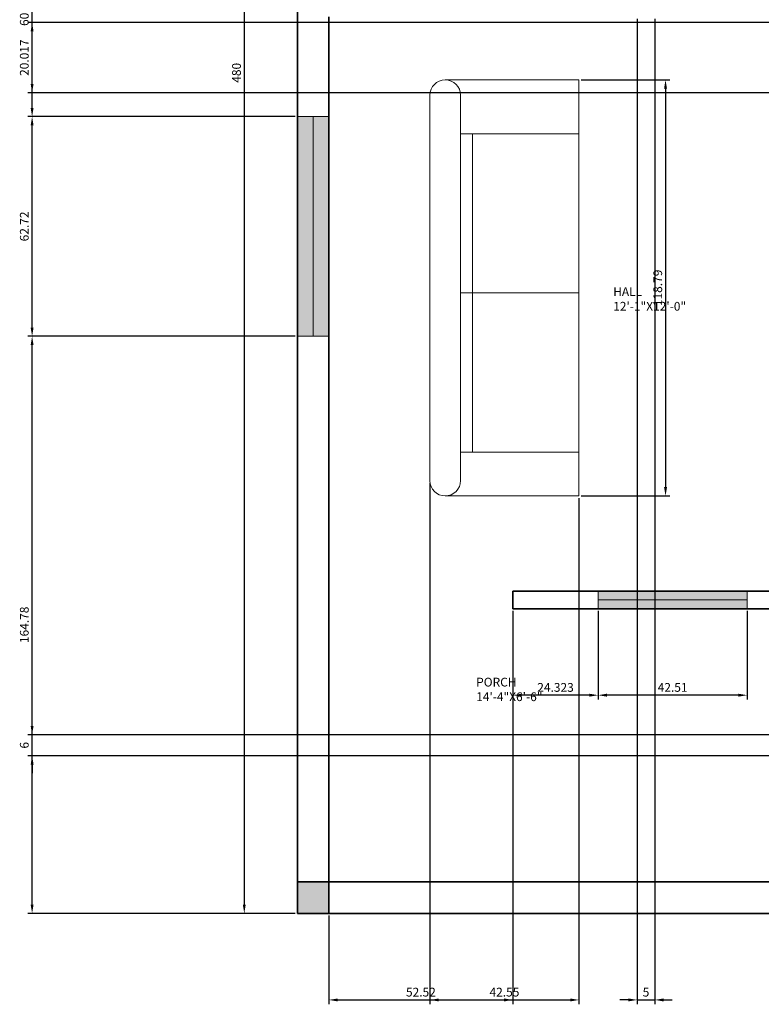
# Model space of a CAD drawing. Units: inches. Extents: x 33934 to 34340, y 20959 to 21493.
# Tile 1 of 4: x 33934 to 34146, y 20959 to 21240. Entities that reach past the tile are written whole.
import ezdxf

# ---------------------------------------------------------------- set-up
doc = ezdxf.new("R2010")
doc.units = ezdxf.units.IN
for name, color, linetype, lineweight in [('A-ANNO-DIMS', 2, 'Continuous', 18), ('A-AREA-IDEN', 7, 'Continuous', 18), ('A-FURN', 8, 'Continuous', 18), ('A-GLAZ', 4, 'Continuous', 18), ('A-WALL', 7, 'Continuous', 35)]:
    doc.layers.add(name, color=color, linetype=linetype, lineweight=lineweight)
doc.layers.add('A-COLS-PATT', color=141, linetype='Continuous', lineweight=13, true_color=0xadddf7)
doc.layers.add('A-GLAZ-PATT', color=159, linetype='Continuous', lineweight=13, true_color=0x22346e)
doc.styles.get("Standard").update_dxf_attribs({"font": 'arial.ttf'})
doc.dimstyles.new('ISO-25', dxfattribs={"dimtxt": 2.5, "dimasz": 2.5, "dimexe": 1.25, "dimexo": 0.625, "dimtad": 1, "dimtxsty": 'Standard', "dimcen": 2.5, "dimadec": 0, "dimazin": 0, "dimtfac": 1, "dimtmove": 0, "dimatfit": 3, "dimfxl": 1, "dimarcsym": 0})

# ---------------------------------------------------------------- blocks, each defined once
blk = doc.blocks.new('*D7')
at = {"layer": 'A-ANNO-DIMS', "color": 0, "lineweight": -2, "transparency": 16777216}
for p, q in [((34013.07, 21465.11), (33997.3, 21465.11)), ((33998.55, 21462.61), (33998.55, 20987.61)), ((34013.07, 20985.11), (33997.3, 20985.11))]:
    blk.add_line(p, q, dxfattribs=at)
at = {"layer": 'A-ANNO-DIMS', "color": 0, "transparency": 16777216}
for points in [[(33998.13, 21462.61), (33998.96, 21462.61), (33998.55, 21465.11)], [(33998.13, 20987.61), (33998.96, 20987.61), (33998.55, 20985.11)]]:
    blk.add_solid(points, dxfattribs=at)
at = {"layer": 'Defpoints', "color": 0, "transparency": 16777216}
for p in [(34013.69, 21465.11), (33998.55, 20985.11), (34013.69, 20985.11)]:
    blk.add_point(p, dxfattribs=at)
at = {"layer": 'A-ANNO-DIMS', "color": 0, "transparency": 16777216, "insert": (33996.64, 21225.11), "char_height": 2.5, "attachment_point": 5, "rotation": 90}
blk.add_mtext('480', dxfattribs=at)
blk = doc.blocks.new('*D17')
at = {"layer": 'A-ANNO-DIMS', "color": 0, "lineweight": -2, "transparency": 16777216}
for p, q in [((34013.07, 21149.89), (33936.74, 21149.89)), ((33937.99, 20987.61), (33937.99, 21147.39)), ((34013.07, 20985.11), (33936.74, 20985.11))]:
    blk.add_line(p, q, dxfattribs=at)
at = {"layer": 'A-ANNO-DIMS', "color": 0, "transparency": 16777216}
for points in [[(33937.58, 21147.39), (33938.41, 21147.39), (33937.99, 21149.89)], [(33937.58, 20987.61), (33938.41, 20987.61), (33937.99, 20985.11)]]:
    blk.add_solid(points, dxfattribs=at)
at = {"layer": 'Defpoints', "color": 0, "transparency": 16777216}
for p in [(33937.99, 21149.89), (34013.69, 21149.89), (34013.69, 20985.11)]:
    blk.add_point(p, dxfattribs=at)
at = {"layer": 'A-ANNO-DIMS', "color": 0, "transparency": 16777216, "insert": (33936.09, 21067.5), "char_height": 2.5, "attachment_point": 5, "rotation": 90}
blk.add_mtext('164.78', dxfattribs=at)
blk = doc.blocks.new('*D18')
at = {"layer": 'A-ANNO-DIMS', "color": 0, "lineweight": -2, "transparency": 16777216}
for p, q in [((34013.07, 21212.61), (33936.74, 21212.61)), ((33937.99, 21152.39), (33937.99, 21210.11)), ((34013.07, 21149.89), (33936.74, 21149.89))]:
    blk.add_line(p, q, dxfattribs=at)
at = {"layer": 'A-ANNO-DIMS', "color": 0, "transparency": 16777216}
for points in [[(33937.58, 21210.11), (33938.41, 21210.11), (33937.99, 21212.61)], [(33937.58, 21152.39), (33938.41, 21152.39), (33937.99, 21149.89)]]:
    blk.add_solid(points, dxfattribs=at)
at = {"layer": 'Defpoints', "color": 0, "transparency": 16777216}
for p in [(33937.99, 21212.61), (34013.69, 21212.61), (34013.69, 21149.89)]:
    blk.add_point(p, dxfattribs=at)
at = {"layer": 'A-ANNO-DIMS', "color": 0, "transparency": 16777216, "insert": (33936.09, 21181.25), "char_height": 2.5, "attachment_point": 5, "rotation": 90}
blk.add_mtext('62.72', dxfattribs=at)
blk = doc.blocks.new('*D19')
at = {"layer": 'A-ANNO-DIMS', "color": 0, "lineweight": -2, "transparency": 16777216}
for p, q in [((34013.07, 21272.89), (33936.74, 21272.89)), ((33937.99, 21215.11), (33937.99, 21270.39)), ((34013.07, 21212.61), (33936.74, 21212.61))]:
    blk.add_line(p, q, dxfattribs=at)
at = {"layer": 'A-ANNO-DIMS', "color": 0, "transparency": 16777216}
for points in [[(33937.58, 21270.39), (33938.41, 21270.39), (33937.99, 21272.89)], [(33937.58, 21215.11), (33938.41, 21215.11), (33937.99, 21212.61)]]:
    blk.add_solid(points, dxfattribs=at)
at = {"layer": 'Defpoints', "color": 0, "transparency": 16777216}
for p in [(33937.99, 21272.89), (34013.69, 21272.89), (34013.69, 21212.61)]:
    blk.add_point(p, dxfattribs=at)
at = {"layer": 'A-ANNO-DIMS', "color": 0, "transparency": 16777216, "insert": (33936.09, 21242.75), "char_height": 2.5, "attachment_point": 5, "rotation": 90}
blk.add_mtext('60.28', dxfattribs=at)
blk = doc.blocks.new('*D32')
at = {"layer": 'A-ANNO-DIMS', "color": 0, "lineweight": -2, "transparency": 16777216}
for p, q in [((33937.99, 21038.61), (33937.99, 21041.11)), ((34167.07, 21036.11), (33936.74, 21036.11)), ((33937.99, 21030.11), (33937.99, 21036.11)), ((34167.07, 21030.11), (33936.74, 21030.11)), ((33937.99, 21027.61), (33937.99, 21025.11))]:
    blk.add_line(p, q, dxfattribs=at)
at = {"layer": 'A-ANNO-DIMS', "color": 0, "transparency": 16777216}
for points in [[(33937.58, 21038.61), (33938.41, 21038.61), (33937.99, 21036.11)], [(33937.58, 21027.61), (33938.41, 21027.61), (33937.99, 21030.11)]]:
    blk.add_solid(points, dxfattribs=at)
at = {"layer": 'Defpoints', "color": 0, "transparency": 16777216}
for p in [(33937.99, 21036.11), (34167.69, 21036.11), (34167.69, 21030.11)]:
    blk.add_point(p, dxfattribs=at)
at = {"layer": 'A-ANNO-DIMS', "color": 0, "transparency": 16777216, "insert": (33936.09, 21033.11), "char_height": 2.5, "attachment_point": 5, "rotation": 90}
blk.add_mtext('6', dxfattribs=at)
blk = doc.blocks.new('*D34')
at = {"layer": 'A-ANNO-DIMS', "color": 0, "lineweight": -2, "transparency": 16777216}
for p, q in [((34051.52, 21108.06), (34051.52, 20959.15)), ((34094.07, 21103.68), (34094.07, 20959.15)), ((34054.02, 20960.4), (34091.57, 20960.4))]:
    blk.add_line(p, q, dxfattribs=at)
at = {"layer": 'A-ANNO-DIMS', "color": 0, "transparency": 16777216}
for points in [[(34054.02, 20960.81), (34054.02, 20959.98), (34051.52, 20960.4)], [(34091.57, 20960.81), (34091.57, 20959.98), (34094.07, 20960.4)]]:
    blk.add_solid(points, dxfattribs=at)
at = {"layer": 'Defpoints', "color": 0, "transparency": 16777216}
for p in [(34051.52, 21108.68), (34094.07, 21104.31), (34094.07, 20960.4)]:
    blk.add_point(p, dxfattribs=at)
at = {"layer": 'A-ANNO-DIMS', "color": 0, "transparency": 16777216, "insert": (34072.79, 20962.3), "char_height": 2.5, "attachment_point": 5}
blk.add_mtext('42.55', dxfattribs=at)
blk = doc.blocks.new('*D35')
at = {"layer": 'A-ANNO-DIMS', "color": 0, "lineweight": -2, "transparency": 16777216}
for p, q in [((34094.69, 21223.1), (34120.02, 21223.1)), ((34118.77, 21220.6), (34118.77, 21106.81)), ((34094.69, 21104.31), (34120.02, 21104.31))]:
    blk.add_line(p, q, dxfattribs=at)
at = {"layer": 'A-ANNO-DIMS', "color": 0, "transparency": 16777216}
for points in [[(34118.35, 21220.6), (34119.19, 21220.6), (34118.77, 21223.1)], [(34118.35, 21106.81), (34119.19, 21106.81), (34118.77, 21104.31)]]:
    blk.add_solid(points, dxfattribs=at)
at = {"layer": 'Defpoints', "color": 0, "transparency": 16777216}
for p in [(34094.07, 21223.1), (34094.07, 21104.31), (34118.77, 21104.31)]:
    blk.add_point(p, dxfattribs=at)
at = {"layer": 'A-ANNO-DIMS', "color": 0, "transparency": 16777216, "insert": (34116.87, 21163.7), "char_height": 2.5, "attachment_point": 5, "rotation": 90}
blk.add_mtext('118.79', dxfattribs=at)
blk = doc.blocks.new('*D37')
at = {"layer": 'A-ANNO-DIMS', "color": 0, "lineweight": -2, "transparency": 16777216}
for p, q in [((34208.35, 21239.44), (33936.74, 21239.44)), ((33937.99, 21221.93), (33937.99, 21236.94)), ((34208.35, 21219.43), (33936.74, 21219.43))]:
    blk.add_line(p, q, dxfattribs=at)
at = {"layer": 'A-ANNO-DIMS', "color": 0, "transparency": 16777216}
for points in [[(33937.58, 21236.94), (33938.41, 21236.94), (33937.99, 21239.44)], [(33937.58, 21221.93), (33938.41, 21221.93), (33937.99, 21219.43)]]:
    blk.add_solid(points, dxfattribs=at)
at = {"layer": 'Defpoints', "color": 0, "transparency": 16777216}
for p in [(33937.99, 21239.44), (34208.98, 21239.44), (34208.98, 21219.43)]:
    blk.add_point(p, dxfattribs=at)
at = {"layer": 'A-ANNO-DIMS', "color": 0, "transparency": 16777216, "insert": (33936.09, 21229.43), "char_height": 2.5, "attachment_point": 5, "rotation": 90}
blk.add_mtext('20.017', dxfattribs=at)
blk = doc.blocks.new('*D38')
at = {"layer": 'A-ANNO-DIMS', "color": 0, "lineweight": -2, "transparency": 16777216}
for p, q in [((34075.21, 21071.49), (34075.21, 21046.16)), ((34099.53, 21071.49), (34099.53, 21046.16)), ((34097.03, 21047.41), (34077.71, 21047.41))]:
    blk.add_line(p, q, dxfattribs=at)
at = {"layer": 'A-ANNO-DIMS', "color": 0, "transparency": 16777216}
for points in [[(34077.71, 21047.83), (34077.71, 21046.99), (34075.21, 21047.41)], [(34097.03, 21047.83), (34097.03, 21046.99), (34099.53, 21047.41)]]:
    blk.add_solid(points, dxfattribs=at)
at = {"layer": 'Defpoints', "color": 0, "transparency": 16777216}
for p in [(34075.21, 21072.11), (34099.53, 21072.11), (34075.21, 21047.41)]:
    blk.add_point(p, dxfattribs=at)
at = {"layer": 'A-ANNO-DIMS', "color": 0, "transparency": 16777216, "insert": (34087.37, 21049.31), "char_height": 2.5, "attachment_point": 5}
blk.add_mtext('24.323', dxfattribs=at)
blk = doc.blocks.new('*D39')
at = {"layer": 'A-ANNO-DIMS', "color": 0, "lineweight": -2, "transparency": 16777216}
for p, q in [((34099.53, 21071.49), (34099.53, 21046.16)), ((34142.05, 21071.49), (34142.05, 21046.16)), ((34139.55, 21047.41), (34102.03, 21047.41))]:
    blk.add_line(p, q, dxfattribs=at)
at = {"layer": 'A-ANNO-DIMS', "color": 0, "transparency": 16777216}
for points in [[(34102.03, 21047.83), (34102.03, 21046.99), (34099.53, 21047.41)], [(34139.55, 21047.83), (34139.55, 21046.99), (34142.05, 21047.41)]]:
    blk.add_solid(points, dxfattribs=at)
at = {"layer": 'Defpoints', "color": 0, "transparency": 16777216}
for p in [(34099.53, 21072.11), (34142.05, 21072.11), (34099.53, 21047.41)]:
    blk.add_point(p, dxfattribs=at)
at = {"layer": 'A-ANNO-DIMS', "color": 0, "transparency": 16777216, "insert": (34120.79, 21049.31), "char_height": 2.5, "attachment_point": 5}
blk.add_mtext('42.51', dxfattribs=at)
blk = doc.blocks.new('*D40')
at = {"layer": 'A-ANNO-DIMS', "color": 0, "lineweight": -2, "transparency": 16777216}
for p, q in [((34075.21, 21071.49), (34075.21, 20959.15)), ((34022.69, 20984.49), (34022.69, 20959.15)), ((34025.19, 20960.4), (34072.71, 20960.4))]:
    blk.add_line(p, q, dxfattribs=at)
at = {"layer": 'A-ANNO-DIMS', "color": 0, "transparency": 16777216}
for points in [[(34025.19, 20960.81), (34025.19, 20959.98), (34022.69, 20960.4)], [(34072.71, 20960.81), (34072.71, 20959.98), (34075.21, 20960.4)]]:
    blk.add_solid(points, dxfattribs=at)
at = {"layer": 'Defpoints', "color": 0, "transparency": 16777216}
for p in [(34075.21, 21072.11), (34022.69, 20985.11), (34075.21, 20960.4)]:
    blk.add_point(p, dxfattribs=at)
at = {"layer": 'A-ANNO-DIMS', "color": 0, "transparency": 16777216, "insert": (34048.95, 20962.3), "char_height": 2.5, "attachment_point": 5}
blk.add_mtext('52.52', dxfattribs=at)
blk = doc.blocks.new('*D51')
at = {"layer": 'A-ANNO-DIMS', "color": 0, "lineweight": -2, "transparency": 16777216}
for p, q in [((34110.69, 21240.49), (34110.69, 20959.15)), ((34115.69, 21240.49), (34115.69, 20959.15)), ((34108.19, 20960.4), (34105.69, 20960.4)), ((34110.69, 20960.4), (34115.69, 20960.4)), ((34118.19, 20960.4), (34120.69, 20960.4))]:
    blk.add_line(p, q, dxfattribs=at)
at = {"layer": 'A-ANNO-DIMS', "color": 0, "transparency": 16777216}
for points in [[(34108.19, 20960.81), (34108.19, 20959.98), (34110.69, 20960.4)], [(34118.19, 20960.81), (34118.19, 20959.98), (34115.69, 20960.4)]]:
    blk.add_solid(points, dxfattribs=at)
at = {"layer": 'Defpoints', "color": 0, "transparency": 16777216}
for p in [(34110.69, 21241.11), (34115.69, 21241.11), (34115.69, 20960.4)]:
    blk.add_point(p, dxfattribs=at)
at = {"layer": 'A-ANNO-DIMS', "color": 0, "transparency": 16777216, "insert": (34113.19, 20962.29), "char_height": 2.5, "attachment_point": 5}
blk.add_mtext('5', dxfattribs=at)

msp = doc.modelspace()

# ---------------------------------------------------------------- hatches: boundary and pattern name
at = {"layer": 'A-COLS-PATT'}
h = msp.add_hatch(color=256, dxfattribs=at)
h.dxf.hatch_style = 1
h.paths.add_polyline_path([(34022.6921, 20994.1104), (34013.6921, 20994.1104), (34013.6921, 20985.1104), (34022.6921, 20985.1104)])
h.paths.add_polyline_path([(34163.6921, 20994.1104), (34158.6922, 20994.1104), (34158.6922, 20985.1104), (34163.6921, 20985.1104)])
h.paths.add_polyline_path([(34313.6921, 20994.1104), (34304.6921, 20994.1104), (34304.6921, 20985.1104), (34313.6921, 20985.1104)])
h.paths.add_polyline_path([(34313.6921, 21077.1104), (34304.6921, 21077.1104), (34304.6921, 21072.1104), (34313.6921, 21072.1104)])
h.paths.add_polyline_path([(34172.6921, 21077.1104), (34167.6921, 21077.1104), (34167.6921, 21072.1104), (34172.6921, 21072.1104)])
h.paths.add_polyline_path([(34022.6921, 21324.1104), (34013.6921, 21324.1104), (34013.6921, 21318.1104), (34022.6921, 21318.1104)])
h.paths.add_polyline_path([(34171.6921, 21324.1104), (34166.6921, 21324.1104), (34166.6921, 21318.1104), (34171.6921, 21318.1104)])
h.paths.add_polyline_path([(34313.6921, 21282.1104), (34304.6921, 21282.1104), (34304.6921, 21277.1104), (34313.6921, 21277.1104)])
h.paths.add_polyline_path([(34313.6921, 21465.1104), (34304.6921, 21465.1104), (34304.6921, 21456.1104), (34313.6921, 21456.1104)])
h.paths.add_polyline_path([(34171.6921, 21465.1104), (34166.6921, 21465.1104), (34166.6921, 21456.1104), (34171.6921, 21456.1104)])
h.paths.add_polyline_path([(34022.6921, 21465.1104), (34013.6921, 21465.1104), (34013.6921, 21456.1104), (34022.6921, 21456.1104)])
at = {"layer": 'A-GLAZ-PATT'}
h = msp.add_hatch(color=256, dxfattribs=at)
h.dxf.hatch_style = 1
h.paths.add_polyline_path([(34022.6921, 21212.6089), (34018.1921, 21212.6089), (34018.1921, 21149.8921), (34022.6921, 21149.8921)])
h.paths.add_polyline_path([(34018.1921, 21212.6089), (34013.6921, 21212.6089), (34013.6921, 21149.8921), (34018.1921, 21149.8921)])
h.paths.add_polyline_path([(34142.0454, 21077.1104), (34099.5314, 21077.1104), (34099.5314, 21074.6104), (34142.0454, 21074.6104)])
h.paths.add_polyline_path([(34142.0454, 21074.6104), (34099.5314, 21074.6104), (34099.5314, 21072.1104), (34142.0454, 21072.1104)])
h.paths.add_polyline_path([(34313.6921, 21160.1148), (34309.1921, 21160.1148), (34309.1921, 21107.9155), (34313.6921, 21107.9155)])
h.paths.add_polyline_path([(34309.1921, 21160.1148), (34304.6921, 21160.1148), (34304.6921, 21107.9155), (34309.1921, 21107.9155)])
h.paths.add_polyline_path([(34309.1921, 21244.1846), (34304.6921, 21244.1846), (34304.6921, 21212.6883), (34309.1921, 21212.6883)])
h.paths.add_polyline_path([(34313.6921, 21244.1846), (34309.1921, 21244.1846), (34309.1921, 21212.6883), (34313.6921, 21212.6883)])
h.paths.add_polyline_path([(34313.6921, 21394.9809), (34309.1921, 21394.9809), (34309.1921, 21355.1902), (34313.6921, 21355.1902)])
h.paths.add_polyline_path([(34309.1921, 21394.9809), (34304.6921, 21394.9809), (34304.6921, 21355.1902), (34309.1921, 21355.1902)])
h.paths.add_polyline_path([(34257.3396, 21465.1104), (34207.5515, 21465.1104), (34207.5515, 21460.6104), (34257.3396, 21460.6104)])
h.paths.add_polyline_path([(34257.3396, 21460.6104), (34207.5515, 21460.6104), (34207.5515, 21456.1104), (34257.3396, 21456.1104)])
h.paths.add_polyline_path([(34117.2268, 21465.1104), (34063.6855, 21465.1104), (34063.6855, 21460.6104), (34117.2268, 21460.6104)])
h.paths.add_polyline_path([(34117.2268, 21460.6104), (34063.6855, 21460.6104), (34063.6855, 21456.1104), (34117.2268, 21456.1104)])
h.paths.add_polyline_path([(34022.6921, 21430.8215), (34018.1921, 21430.8215), (34018.1921, 21373.469), (34022.6921, 21373.469)])
h.paths.add_polyline_path([(34018.1921, 21430.8215), (34013.6921, 21430.8215), (34013.6921, 21373.469), (34018.1921, 21373.469)])
h.paths.add_polyline_path([(34018.1921, 21305.2021), (34013.6921, 21305.2021), (34013.6921, 21272.8905), (34018.1921, 21272.8905)])
h.paths.add_polyline_path([(34022.6921, 21305.2021), (34018.1921, 21305.2021), (34018.1921, 21272.8905), (34022.6921, 21272.8905)])

# ---------------------------------------------------------------- linework, layer by layer
at = {"layer": 'A-FURN'}
for p, q in [((34055.8927, 21223.0953), (34094.0686, 21223.0953)), ((34094.0686, 21223.0953), (34094.0686, 21207.6614)), ((34051.5214, 21108.6803), (34051.5214, 21218.724)), ((34060.2639, 21218.724), (34060.2639, 21108.6803)), ((34060.2639, 21207.6614), (34094.0686, 21207.6614)), ((34060.2639, 21116.8317), (34060.2639, 21207.6614)), ((34063.6318, 21116.8317), (34063.6318, 21207.6614)), ((34094.0686, 21207.6614), (34094.0686, 21116.8317)), ((34094.0686, 21162.2465), (34060.2639, 21162.2465)), ((34094.0686, 21116.8317), (34060.2639, 21116.8317)), ((34094.0686, 21104.309), (34094.0686, 21116.8317)), ((34055.8927, 21104.309), (34094.0686, 21104.309))]:
    msp.add_line(p, q, dxfattribs=at)
for centre, start, end in [((34055.8927, 21218.724), 0, 180), ((34055.8927, 21108.6803), 180, 0)]:
    msp.add_arc(centre, 4.3713, start, end, dxfattribs=at)
at = {"layer": 'A-GLAZ'}
for p, q in [((34022.6921, 21212.6089), (34013.6921, 21212.6089)), ((34013.6921, 21212.6089), (34013.6921, 21149.8921)), ((34018.1921, 21149.8921), (34018.1921, 21212.6089)), ((34013.6921, 21149.8921), (34022.6921, 21149.8921)), ((34022.6921, 21149.8921), (34018.1921, 21149.8921)), ((34099.5314, 21072.1104), (34099.5314, 21077.1104)), ((34099.5314, 21077.1104), (34142.0454, 21077.1104)), ((34142.0454, 21077.1104), (34142.0454, 21072.1104)), ((34142.0454, 21077.1104), (34142.0454, 21074.6104)), ((34142.0454, 21074.6104), (34099.5314, 21074.6104)), ((34142.0454, 21072.1104), (34099.5314, 21072.1104))]:
    msp.add_line(p, q, dxfattribs=at)
at = {"layer": 'A-WALL'}
for p, q in [((34013.6921, 20985.1104), (34013.6921, 21465.1104)), ((34022.6921, 20985.1104), (34022.6921, 21241.1104)), ((34075.2088, 21077.1104), (34075.2088, 21072.1104)), ((34167.6921, 21077.1104), (34075.2088, 21077.1104)), ((34313.6921, 21072.1104), (34075.2088, 21072.1104)), ((34313.6921, 20994.1104), (34013.6921, 20994.1104)), ((34313.6921, 20985.1104), (34013.6921, 20985.1104))]:
    msp.add_line(p, q, dxfattribs=at)

# ---------------------------------------------------------------- texts
at = {"layer": 'A-AREA-IDEN', "char_height": 2.5, "attachment_point": 1}
for s, width, insert in [('HALL\\P12\'-1"X12\'-0"', 30.559255, (34103.8295, 21163.8672)), ('PORCH\\P14\'-4"X6\'-6"', 79.851846, (34064.7229, 21052.3871))]:
    msp.add_mtext_dynamic_manual_height_columns(s, width=width, gutter_width=12.5, heights=[0], dxfattribs=dict(at, insert=insert))

# ---------------------------------------------------------------- dimensions: what is measured, and where the dimension line sits
at = {"layer": 'A-ANNO-DIMS'}
for base, p1, p2, angle, override, picture, middle in [((33998.546, 20985.1104), (34013.6921, 21465.1104), (34013.6921, 20985.1104), 90, {"dimclrd": 0, "dimclre": 0, "dimclrt": 0}, '*D7', (33996.6445, 21225.1104)), ((33937.9921, 21272.8905), (34013.6921, 21212.6089), (34013.6921, 21272.8905), 90, {"dimdec": 2, "dimlfac": 1, "dimrnd": 0, "dimzin": 0, "dimdsep": 46, "dimlunit": 2}, '*D19', (33936.0907, 21242.7497)), ((33937.9921, 21239.4434), (34208.9796, 21219.4265), (34208.9796, 21239.4434), 90, {"dimdec": 3, "dimlfac": 1, "dimrnd": 0, "dimzin": 0, "dimdsep": 46, "dimlunit": 2}, '*D37', (33936.0907, 21229.4349)), ((34118.7686, 21104.309), (34094.0686, 21223.0953), (34094.0686, 21104.309), 270, {"dimdec": 2, "dimlfac": 1, "dimrnd": 0, "dimzin": 0, "dimdsep": 46, "dimlunit": 2}, '*D35', (34116.8671, 21163.7021)), ((33937.9921, 21212.6089), (34013.6921, 21149.8921), (34013.6921, 21212.6089), 90, {"dimdec": 2, "dimlfac": 1, "dimrnd": 0, "dimzin": 0, "dimdsep": 46, "dimlunit": 2}, '*D18', (33936.0907, 21181.2505)), ((33937.9921, 21149.8921), (34013.6921, 20985.1104), (34013.6921, 21149.8921), 90, {"dimdec": 2, "dimlfac": 1, "dimrnd": 0, "dimzin": 0, "dimdsep": 46, "dimlunit": 2}, '*D17', (33936.0907, 21067.5013)), ((34075.2088, 21047.4104), (34099.5314, 21072.1104), (34075.2088, 21072.1104), 180, {"dimdec": 3, "dimlfac": 1, "dimrnd": 0, "dimzin": 0, "dimdsep": 46, "dimlunit": 2}, '*D38', (34087.3701, 21049.3127)), ((34099.5314, 21047.4104), (34142.0454, 21072.1104), (34099.5314, 21072.1104), 180, {"dimdec": 2, "dimlfac": 1, "dimrnd": 0, "dimzin": 0, "dimdsep": 46, "dimlunit": 2}, '*D39', (34120.7884, 21049.3119)), ((33937.9921, 21036.1104), (34167.6921, 21030.1104), (34167.6921, 21036.1104), 90, {"dimdec": 0, "dimlfac": 1, "dimrnd": 0, "dimzin": 0, "dimdsep": 46, "dimlunit": 2}, '*D32', (33936.0907, 21033.1104))]:
    dim = msp.add_linear_dim(base=base, p1=p1, p2=p2, angle=angle, dimstyle='ISO-25', override=override, dxfattribs=at)
    dim.commit()
    dim.dimension.update_dxf_attribs({"geometry": picture, "text_midpoint": middle})
for base, p1, p2, override, picture, middle in [((34115.6921, 20960.3981), (34110.6921, 21241.1104), (34115.6921, 21241.1104), {"dimdec": 0, "dimlfac": 1, "dimrnd": 0, "dimzin": 0, "dimdsep": 46, "dimlunit": 2}, '*D51', (34113.1921, 20962.2944)), ((34094.0686, 20960.3981), (34051.5214, 21108.6803), (34094.0686, 21104.309), {"dimdec": 2, "dimlfac": 1, "dimrnd": 0, "dimzin": 0, "dimdsep": 46, "dimlunit": 2}, '*D34', (34072.795, 20962.2995)), ((34075.2088, 20960.3981), (34022.6921, 20985.1104), (34075.2088, 21072.1104), {"dimdec": 2, "dimlfac": 1, "dimrnd": 0, "dimzin": 0, "dimdsep": 46, "dimlunit": 2}, '*D40', (34048.9505, 20962.2995))]:
    dim = msp.add_linear_dim(base=base, p1=p1, p2=p2, dimstyle='ISO-25', override=override, dxfattribs=at)
    dim.commit()
    dim.dimension.update_dxf_attribs({"geometry": picture, "text_midpoint": middle})

doc.saveas('drawing.dxf')
